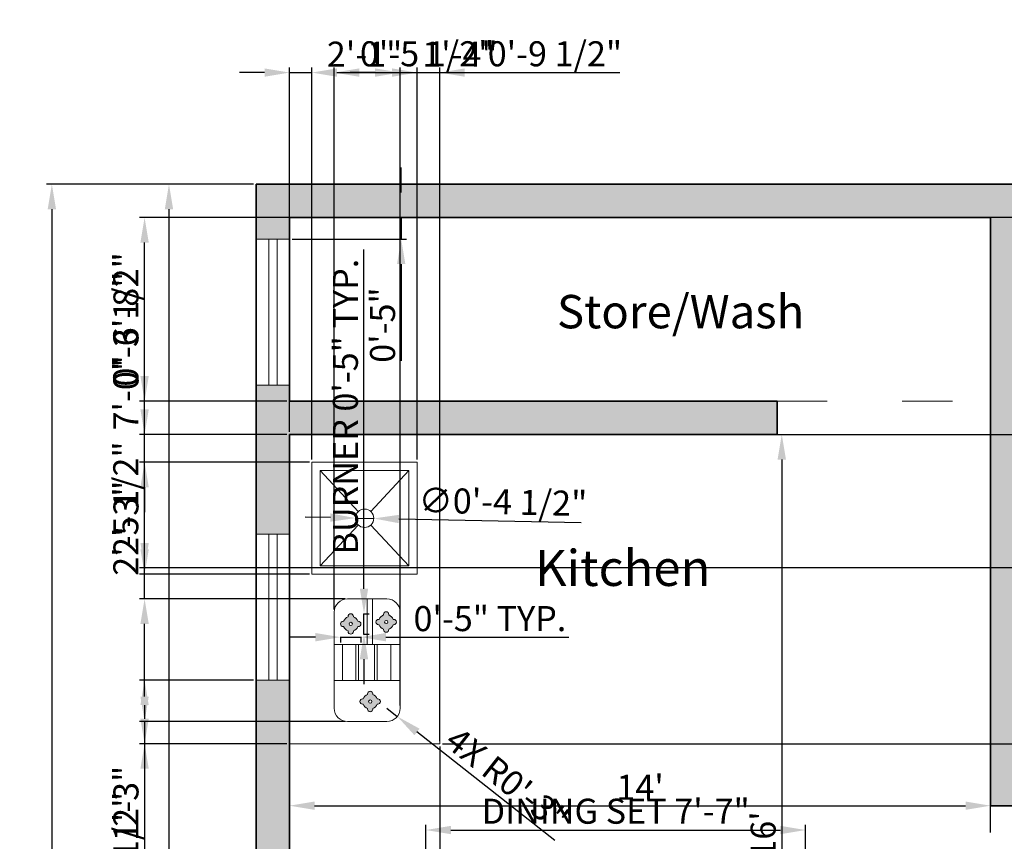
# Model space of a CAD drawing. Units: inches. Extents: x 2129 to 3258, y 1851 to 3021.
# Tile 6 of 10: x 2129 to 2365, y 2250 to 2447. Entities that reach past the tile are written whole.
import ezdxf

# ---------------------------------------------------------------- set-up
doc = ezdxf.new("R2010")
doc.units = ezdxf.units.IN
doc.linetypes.add('ACAD_ISO03W100', pattern=[30, 12, -18])
for name, color, linetype, lineweight in [('A-ANNO-DIMS', 2, 'Continuous', 18), ('A-AREA-IDEN', 7, 'Continuous', 20), ('A-EQPM', 4, 'Continuous', 13), ('A-FLOR-CASE', 8, 'Continuous', 18), ('A-FLOR-FIXT', 9, 'Continuous', 18), ('A-GLAZ', 4, 'Continuous', 18), ('A-WALL', 7, 'Continuous', 35), ('A-WALL-OVHD', 8, 'ACAD_ISO03W100', 18)]:
    doc.layers.add(name, color=color, linetype=linetype, lineweight=lineweight)
doc.layers.add('A-WALL-PATT', color=32, linetype='Continuous', lineweight=13, true_color=0xcd6928)
doc.styles.get("Standard").update_dxf_attribs({"font": 'arial.ttf'})
doc.dimstyles.new('ISO-25', dxfattribs={"dimtxt": 6, "dimasz": 6, "dimexe": 1.25, "dimexo": 0.625, "dimtad": 1, "dimdec": 1, "dimlunit": 3, "dimtxsty": 'Standard', "dimcen": 2.5, "dimclrd": 5, "dimclre": 5, "dimadec": 0, "dimazin": 0, "dimtfac": 1, "dimtdec": 1, "dimtmove": 0, "dimatfit": 3, "dimfxl": 1, "dimarcsym": 0})

# ---------------------------------------------------------------- blocks, each defined once
blk = doc.blocks.new('*D5')
at = {"layer": 'A-ANNO-DIMS', "color": 0, "lineweight": -2, "transparency": 16777216}
for p, q in [((2185.3, 2407.23), (2163.77, 2407.23)), ((2165.02, 2401.23), (2165.02, 1965.23)), ((2185.3, 1959.23), (2163.77, 1959.23))]:
    blk.add_line(p, q, dxfattribs=at)
at = {"layer": 'A-ANNO-DIMS', "color": 0, "transparency": 16777216}
for points in [[(2164.02, 2401.23), (2166.02, 2401.23), (2165.02, 2407.23)], [(2164.02, 1965.23), (2166.02, 1965.23), (2165.02, 1959.23)]]:
    blk.add_solid(points, dxfattribs=at)
at = {"layer": 'Defpoints', "color": 0, "transparency": 16777216}
for p in [(2185.93, 2407.23), (2165.02, 1959.23), (2185.93, 1959.23)]:
    blk.add_point(p, dxfattribs=at)
at = {"layer": 'A-ANNO-DIMS', "color": 0, "transparency": 16777216, "insert": (2161.33, 2183.23), "char_height": 6, "attachment_point": 5, "rotation": 90}
blk.add_mtext('37\'-4"', dxfattribs=at)
blk = doc.blocks.new('*D6')
at = {"layer": 'A-ANNO-DIMS', "color": 0, "lineweight": -2, "transparency": 16777216}
for p, q in [((2185.3, 2407.23), (2135.71, 2407.23)), ((2136.96, 2401.23), (2136.96, 1885.23)), ((2185.3, 1879.23), (2135.71, 1879.23))]:
    blk.add_line(p, q, dxfattribs=at)
at = {"layer": 'A-ANNO-DIMS', "color": 0, "transparency": 16777216}
for points in [[(2135.96, 2401.23), (2137.96, 2401.23), (2136.96, 2407.23)], [(2135.96, 1885.23), (2137.96, 1885.23), (2136.96, 1879.23)]]:
    blk.add_solid(points, dxfattribs=at)
at = {"layer": 'Defpoints', "color": 0, "transparency": 16777216}
for p in [(2185.93, 2407.23), (2136.96, 1879.23), (2185.93, 1879.23)]:
    blk.add_point(p, dxfattribs=at)
at = {"layer": 'A-ANNO-DIMS', "color": 0, "transparency": 16777216, "insert": (2133.34, 2143.23), "char_height": 6, "attachment_point": 5, "rotation": 90}
blk.add_mtext("44'", dxfattribs=at)
blk = doc.blocks.new('*D7')
at = {"layer": 'A-ANNO-DIMS', "color": 0, "lineweight": -2, "transparency": 16777216}
for p, q in [((2311.4, 2347.23), (2313.14, 2347.23)), ((2311.89, 2341.23), (2311.89, 2161.23)), ((2311.4, 2155.23), (2313.14, 2155.23))]:
    blk.add_line(p, q, dxfattribs=at)
at = {"layer": 'A-ANNO-DIMS', "color": 0, "transparency": 16777216}
for points in [[(2310.89, 2341.23), (2312.89, 2341.23), (2311.89, 2347.23)], [(2310.89, 2161.23), (2312.89, 2161.23), (2311.89, 2155.23)]]:
    blk.add_solid(points, dxfattribs=at)
at = {"layer": 'Defpoints', "color": 0, "transparency": 16777216}
for p in [(2310.77, 2347.23), (2310.77, 2155.23), (2311.89, 2155.23)]:
    blk.add_point(p, dxfattribs=at)
at = {"layer": 'A-ANNO-DIMS', "color": 0, "transparency": 16777216, "insert": (2308.2, 2251.23), "char_height": 6, "attachment_point": 5, "rotation": 90}
blk.add_mtext("16'", dxfattribs=at)
blk = doc.blocks.new('*D8')
at = {"layer": 'A-ANNO-DIMS', "color": 0, "lineweight": -2, "transparency": 16777216}
for p, q in [((2193.93, 2251.86), (2193.93, 2259.5)), ((2361.93, 2251.86), (2361.93, 2259.5)), ((2199.93, 2258.25), (2355.93, 2258.25))]:
    blk.add_line(p, q, dxfattribs=at)
at = {"layer": 'A-ANNO-DIMS', "color": 0, "transparency": 16777216}
for points in [[(2199.93, 2259.25), (2199.93, 2257.25), (2193.93, 2258.25)], [(2355.93, 2259.25), (2355.93, 2257.25), (2361.93, 2258.25)]]:
    blk.add_solid(points, dxfattribs=at)
at = {"layer": 'Defpoints', "color": 0, "transparency": 16777216}
for p in [(2361.93, 2258.25), (2193.93, 2251.23), (2361.93, 2251.23)]:
    blk.add_point(p, dxfattribs=at)
at = {"layer": 'A-ANNO-DIMS', "color": 0, "transparency": 16777216, "insert": (2277.93, 2261.89), "char_height": 6, "attachment_point": 5}
blk.add_mtext("14'", dxfattribs=at)
blk = doc.blocks.new('WIN-PLAN-35')
for p, q in [((0, 5), (35, 5)), ((0, 3), (35, 3))]:
    blk.add_line(p, q)
blk.add_lwpolyline([(0, 8), (35, 8), (35, 0), (0, 0)], close=True)
blk = doc.blocks.new('COOKTOP-BURNER')
h = blk.add_hatch(color=256)
h.dxf.hatch_style = 1
h.paths.add_polyline_path([(0.76, 3.09), (0.64, 3.09, 1), (0.64, 1.81), (0.76, 1.81, 0.214506), (1.81, 0.76), (1.81, 0.64, 1), (3.09, 0.64), (3.09, 0.76, 0.214506), (4.14, 1.81), (4.26, 1.81, 1), (4.26, 3.09), (4.14, 3.09, 0.214506), (3.09, 4.14), (3.09, 4.26, 1), (1.81, 4.26), (1.81, 4.14, 0.214506)])
h.paths.add_polyline_path([(2.45, 2.84, -1), (2.45, 2.06, -1)], flags=16)
for p, q in [((0.64, 3.09), (0.76, 3.09)), ((1.81, 4.14), (1.81, 4.26)), ((3.09, 4.14), (3.09, 4.26)), ((4.14, 3.09), (4.26, 3.09)), ((0.64, 1.81), (0.76, 1.81)), ((1.81, 0.64), (1.81, 0.76)), ((3.09, 0.64), (3.09, 0.76)), ((4.14, 1.81), (4.26, 1.81))]:
    blk.add_line(p, q)
blk.add_circle((2.45, 2.45), 0.392)
for centre, radius, start, end in [((2.45, 4.26), 0.642, 0, 180), ((0.64, 2.45), 0.642, 90, 270), ((2.45, 2.45), 1.81, 110.7864, 159.2136), ((2.45, 2.45), 1.81, 20.7864, 69.2136), ((4.26, 2.45), 0.642, 270, 90), ((2.45, 2.45), 1.81, 200.7864, 249.2136), ((2.45, 0.64), 0.642, 180, 0), ((2.45, 2.45), 1.81, 290.7864, 339.2136)]:
    blk.add_arc(centre, radius, start, end)
blk = doc.blocks.new('*D70')
at = {"layer": 'A-ANNO-DIMS', "color": 5, "lineweight": -2, "transparency": 16777216}
for p, q in [((2211.76, 2310.27), (2211.76, 2391.55)), ((2211.65, 2304.27), (2213.01, 2304.27)), ((2211.76, 2299.37), (2211.76, 2304.27)), ((2211.65, 2299.37), (2213.01, 2299.37)), ((2211.76, 2293.37), (2211.76, 2287.37))]:
    blk.add_line(p, q, dxfattribs=at)
at = {"layer": 'A-ANNO-DIMS', "color": 5, "transparency": 16777216}
for points in [[(2210.76, 2310.27), (2212.76, 2310.27), (2211.76, 2304.27)], [(2210.76, 2293.37), (2212.76, 2293.37), (2211.76, 2299.37)]]:
    blk.add_solid(points, dxfattribs=at)
at = {"layer": 'Defpoints', "color": 0, "transparency": 16777216}
for p in [(2211.03, 2304.27), (2211.76, 2304.27), (2211.03, 2299.37)]:
    blk.add_point(p, dxfattribs=at)
at = {"layer": 'A-ANNO-DIMS', "color": 0, "transparency": 16777216, "insert": (2208.08, 2353.91), "char_height": 6, "attachment_point": 5, "rotation": 90}
blk.add_mtext('BURNER 0\'-5" TYP.', dxfattribs=at)
blk = doc.blocks.new('*D71')
at = {"layer": 'A-ANNO-DIMS', "color": 5, "lineweight": -2, "transparency": 16777216}
for p, q in [((2200.13, 2298.64), (2194.13, 2298.64)), ((2206.13, 2298.75), (2206.13, 2297.39)), ((2206.13, 2298.64), (2211.03, 2298.64)), ((2211.03, 2298.75), (2211.03, 2297.39)), ((2217.03, 2298.64), (2260.85, 2298.64))]:
    blk.add_line(p, q, dxfattribs=at)
at = {"layer": 'A-ANNO-DIMS', "color": 5, "transparency": 16777216}
for points in [[(2200.13, 2299.64), (2200.13, 2297.64), (2206.13, 2298.64)], [(2217.03, 2299.64), (2217.03, 2297.64), (2211.03, 2298.64)]]:
    blk.add_solid(points, dxfattribs=at)
at = {"layer": 'Defpoints', "color": 0, "transparency": 16777216}
for p in [(2206.13, 2299.37), (2211.03, 2299.37), (2211.03, 2298.64)]:
    blk.add_point(p, dxfattribs=at)
at = {"layer": 'A-ANNO-DIMS', "color": 0, "transparency": 16777216, "insert": (2241.94, 2302.32), "char_height": 6, "attachment_point": 5}
blk.add_mtext('0\'-5" TYP.', dxfattribs=at)
blk = doc.blocks.new('*D78')
at = {"layer": 'A-ANNO-DIMS', "color": 5, "lineweight": -2, "transparency": 16777216}
for p, q in [((2226.58, 2239.39), (2226.58, 2253.67)), ((2317.58, 2239.39), (2317.58, 2253.67)), ((2232.58, 2252.42), (2311.58, 2252.42))]:
    blk.add_line(p, q, dxfattribs=at)
at = {"layer": 'A-ANNO-DIMS', "color": 5, "transparency": 16777216}
for points in [[(2232.58, 2253.42), (2232.58, 2251.42), (2226.58, 2252.42)], [(2311.58, 2253.42), (2311.58, 2251.42), (2317.58, 2252.42)]]:
    blk.add_solid(points, dxfattribs=at)
at = {"layer": 'Defpoints', "color": 0, "transparency": 16777216}
for p in [(2317.58, 2252.42), (2226.58, 2238.77), (2317.58, 2238.77)]:
    blk.add_point(p, dxfattribs=at)
at = {"layer": 'A-ANNO-DIMS', "color": 0, "transparency": 16777216, "insert": (2272.08, 2256.15), "char_height": 6, "attachment_point": 5}
blk.add_mtext('DINING SET 7\'-7"', dxfattribs=at)
blk = doc.blocks.new('*D92')
at = {"layer": 'A-ANNO-DIMS', "color": 5, "lineweight": -2, "transparency": 16777216}
for p, q in [((2369.3, 2399.23), (2157.93, 2399.23)), ((2159.18, 2321.23), (2159.18, 2393.23)), ((2369.3, 2315.23), (2157.93, 2315.23))]:
    blk.add_line(p, q, dxfattribs=at)
at = {"layer": 'A-ANNO-DIMS', "color": 5, "transparency": 16777216}
for points in [[(2158.18, 2393.23), (2160.18, 2393.23), (2159.18, 2399.23)], [(2158.18, 2321.23), (2160.18, 2321.23), (2159.18, 2315.23)]]:
    blk.add_solid(points, dxfattribs=at)
at = {"layer": 'Defpoints', "color": 0, "transparency": 16777216}
for p in [(2159.18, 2399.23), (2369.93, 2399.23), (2369.93, 2315.23)]:
    blk.add_point(p, dxfattribs=at)
at = {"layer": 'A-ANNO-DIMS', "color": 0, "transparency": 16777216, "insert": (2155.49, 2357.23), "char_height": 6, "attachment_point": 5, "rotation": 90}
blk.add_mtext('7\'-0"', dxfattribs=at)
blk = doc.blocks.new('*D93')
at = {"layer": 'A-ANNO-DIMS', "color": 5, "lineweight": -2, "transparency": 16777216}
for p, q in [((2193.3, 2399.23), (2157.93, 2399.23)), ((2159.18, 2361.23), (2159.18, 2393.23)), ((2193.3, 2355.23), (2157.93, 2355.23))]:
    blk.add_line(p, q, dxfattribs=at)
at = {"layer": 'A-ANNO-DIMS', "color": 5, "transparency": 16777216}
for points in [[(2158.18, 2393.23), (2160.18, 2393.23), (2159.18, 2399.23)], [(2158.18, 2361.23), (2160.18, 2361.23), (2159.18, 2355.23)]]:
    blk.add_solid(points, dxfattribs=at)
at = {"layer": 'Defpoints', "color": 0, "transparency": 16777216}
for p in [(2159.18, 2399.23), (2193.93, 2399.23), (2193.93, 2355.23)]:
    blk.add_point(p, dxfattribs=at)
at = {"layer": 'A-ANNO-DIMS', "color": 0, "transparency": 16777216, "insert": (2155.49, 2377.23), "char_height": 6, "attachment_point": 5, "rotation": 90}
blk.add_mtext('3\'-8"', dxfattribs=at)
blk = doc.blocks.new('*D97')
at = {"layer": 'A-ANNO-DIMS', "color": 5, "lineweight": -2, "transparency": 16777216}
for p, q in [((2193.93, 2272.48), (2193.93, 1851.23)), ((2229.93, 2272.48), (2229.93, 1851.23)), ((2199.93, 1852.48), (2223.93, 1852.48))]:
    blk.add_line(p, q, dxfattribs=at)
at = {"layer": 'A-ANNO-DIMS', "color": 5, "transparency": 16777216}
for points in [[(2199.93, 1853.48), (2199.93, 1851.48), (2193.93, 1852.48)], [(2223.93, 1853.48), (2223.93, 1851.48), (2229.93, 1852.48)]]:
    blk.add_solid(points, dxfattribs=at)
at = {"layer": 'Defpoints', "color": 0, "transparency": 16777216}
for p in [(2193.93, 2273.1), (2229.93, 2273.1), (2229.93, 1852.48)]:
    blk.add_point(p, dxfattribs=at)
at = {"layer": 'A-ANNO-DIMS', "color": 0, "transparency": 16777216, "insert": (2211.93, 1856.18), "char_height": 6, "attachment_point": 5}
blk.add_mtext('3\'-0"', dxfattribs=at)
blk = doc.blocks.new('*D98')
at = {"layer": 'A-ANNO-DIMS', "color": 5, "lineweight": -2, "transparency": 16777216}
for p, q in [((2230.55, 2347.23), (2597.93, 2347.23)), ((2596.68, 2279.1), (2596.68, 2341.23)), ((2230.55, 2273.1), (2597.93, 2273.1))]:
    blk.add_line(p, q, dxfattribs=at)
at = {"layer": 'A-ANNO-DIMS', "color": 5, "transparency": 16777216}
for points in [[(2595.68, 2341.23), (2597.68, 2341.23), (2596.68, 2347.23)], [(2595.68, 2279.1), (2597.68, 2279.1), (2596.68, 2273.1)]]:
    blk.add_solid(points, dxfattribs=at)
at = {"layer": 'Defpoints', "color": 0, "transparency": 16777216}
for p in [(2229.93, 2347.23), (2596.68, 2347.23), (2229.93, 2273.1)]:
    blk.add_point(p, dxfattribs=at)
at = {"layer": 'A-ANNO-DIMS', "color": 0, "transparency": 16777216, "insert": (2592.99, 2310.17), "char_height": 6, "attachment_point": 5, "rotation": 90}
blk.add_mtext('6\'-2"', dxfattribs=at)
blk = doc.blocks.new('*D99')
at = {"layer": 'A-ANNO-DIMS', "color": 5, "lineweight": -2, "transparency": 16777216}
for p, q in [((2199.29, 2341.21), (2199.29, 2435.23)), ((2205.29, 2433.98), (2218.51, 2433.98)), ((2224.51, 2341.21), (2224.51, 2435.23))]:
    blk.add_line(p, q, dxfattribs=at)
at = {"layer": 'A-ANNO-DIMS', "color": 5, "transparency": 16777216}
for points in [[(2205.29, 2434.98), (2205.29, 2432.98), (2199.29, 2433.98)], [(2218.51, 2434.98), (2218.51, 2432.98), (2224.51, 2433.98)]]:
    blk.add_solid(points, dxfattribs=at)
at = {"layer": 'Defpoints', "color": 0, "transparency": 16777216}
for p in [(2224.51, 2433.98), (2199.29, 2340.59), (2224.51, 2340.59)]:
    blk.add_point(p, dxfattribs=at)
at = {"layer": 'A-ANNO-DIMS', "color": 0, "transparency": 16777216, "insert": (2211.9, 2437.62), "char_height": 6, "attachment_point": 5}
blk.add_mtext('2\'-1"', dxfattribs=at)
blk = doc.blocks.new('*D100')
at = {"layer": 'A-ANNO-DIMS', "color": 5, "lineweight": -2, "transparency": 16777216}
for p, q in [((2198.67, 2340.59), (2157.93, 2340.59)), ((2159.18, 2319.71), (2159.18, 2334.59)), ((2198.67, 2313.71), (2157.93, 2313.71))]:
    blk.add_line(p, q, dxfattribs=at)
at = {"layer": 'A-ANNO-DIMS', "color": 5, "transparency": 16777216}
for points in [[(2158.18, 2334.59), (2160.18, 2334.59), (2159.18, 2340.59)], [(2158.18, 2319.71), (2160.18, 2319.71), (2159.18, 2313.71)]]:
    blk.add_solid(points, dxfattribs=at)
at = {"layer": 'Defpoints', "color": 0, "transparency": 16777216}
for p in [(2159.18, 2340.59), (2199.29, 2340.59), (2199.29, 2313.71)]:
    blk.add_point(p, dxfattribs=at)
at = {"layer": 'A-ANNO-DIMS', "color": 0, "transparency": 16777216, "insert": (2155.49, 2327.15), "char_height": 6, "attachment_point": 5, "rotation": 90}
blk.add_mtext('2\'-3"', dxfattribs=at)
blk = doc.blocks.new('*D101')
at = {"layer": 'A-ANNO-DIMS', "color": 5, "lineweight": -2, "transparency": 16777216}
for p, q in [((2204.64, 2305.25), (2204.64, 2435.23)), ((2210.64, 2433.98), (2214.44, 2433.98)), ((2220.44, 2305.25), (2220.44, 2435.23)), ((2220.44, 2433.98), (2243.07, 2433.98))]:
    blk.add_line(p, q, dxfattribs=at)
at = {"layer": 'A-ANNO-DIMS', "color": 5, "transparency": 16777216}
for points in [[(2210.64, 2434.98), (2210.64, 2432.98), (2204.64, 2433.98)], [(2214.44, 2434.98), (2214.44, 2432.98), (2220.44, 2433.98)]]:
    blk.add_solid(points, dxfattribs=at)
at = {"layer": 'Defpoints', "color": 0, "transparency": 16777216}
for p in [(2220.44, 2433.98), (2204.64, 2304.63), (2220.44, 2304.63)]:
    blk.add_point(p, dxfattribs=at)
at = {"layer": 'A-ANNO-DIMS', "color": 0, "transparency": 16777216, "insert": (2234.76, 2437.62), "char_height": 6, "attachment_point": 5}
blk.add_mtext('1\'-4"', dxfattribs=at)
blk = doc.blocks.new('*D102')
at = {"layer": 'A-ANNO-DIMS', "color": 5, "lineweight": -2, "transparency": 16777216}
for p, q in [((2159.18, 2307.84), (2159.18, 2345.12)), ((2207.23, 2307.84), (2157.93, 2307.84)), ((2159.18, 2284.42), (2159.18, 2301.84)), ((2207.23, 2278.42), (2157.93, 2278.42))]:
    blk.add_line(p, q, dxfattribs=at)
at = {"layer": 'A-ANNO-DIMS', "color": 5, "transparency": 16777216}
for points in [[(2158.18, 2301.84), (2160.18, 2301.84), (2159.18, 2307.84)], [(2158.18, 2284.42), (2160.18, 2284.42), (2159.18, 2278.42)]]:
    blk.add_solid(points, dxfattribs=at)
at = {"layer": 'Defpoints', "color": 0, "transparency": 16777216}
for p in [(2159.18, 2307.84), (2207.85, 2307.84), (2207.85, 2278.42)]:
    blk.add_point(p, dxfattribs=at)
at = {"layer": 'A-ANNO-DIMS', "color": 0, "transparency": 16777216, "insert": (2155.45, 2329.48), "char_height": 6, "attachment_point": 5, "rotation": 90}
blk.add_mtext('2\'-5 1/2"', dxfattribs=at)
blk = doc.blocks.new('*D103')
at = {"layer": 'A-ANNO-DIMS', "color": 5, "lineweight": -2, "transparency": 16777216}
for p, q in [((2187.93, 2433.98), (2181.93, 2433.98)), ((2193.93, 2347.86), (2193.93, 2435.23)), ((2193.93, 2433.98), (2199.29, 2433.98)), ((2199.29, 2341.21), (2199.29, 2435.23)), ((2205.29, 2433.98), (2242.47, 2433.98))]:
    blk.add_line(p, q, dxfattribs=at)
at = {"layer": 'A-ANNO-DIMS', "color": 5, "transparency": 16777216}
for points in [[(2187.93, 2434.98), (2187.93, 2432.98), (2193.93, 2433.98)], [(2205.29, 2434.98), (2205.29, 2432.98), (2199.29, 2433.98)]]:
    blk.add_solid(points, dxfattribs=at)
at = {"layer": 'Defpoints', "color": 0, "transparency": 16777216}
for p in [(2199.29, 2433.98), (2193.93, 2347.23), (2199.29, 2340.59)]:
    blk.add_point(p, dxfattribs=at)
at = {"layer": 'A-ANNO-DIMS', "color": 0, "transparency": 16777216, "insert": (2226.88, 2437.71), "char_height": 6, "attachment_point": 5}
blk.add_mtext('0\'-5 1/2"', dxfattribs=at)
blk = doc.blocks.new('*D104')
at = {"layer": 'A-ANNO-DIMS', "color": 5, "lineweight": -2, "transparency": 16777216}
for p, q in [((2159.18, 2353.23), (2159.18, 2390.42)), ((2193.3, 2347.23), (2157.93, 2347.23)), ((2159.18, 2340.59), (2159.18, 2347.23)), ((2198.67, 2340.59), (2157.93, 2340.59)), ((2159.18, 2334.59), (2159.18, 2328.59))]:
    blk.add_line(p, q, dxfattribs=at)
at = {"layer": 'A-ANNO-DIMS', "color": 5, "transparency": 16777216}
for points in [[(2158.18, 2353.23), (2160.18, 2353.23), (2159.18, 2347.23)], [(2158.18, 2334.59), (2160.18, 2334.59), (2159.18, 2340.59)]]:
    blk.add_solid(points, dxfattribs=at)
at = {"layer": 'Defpoints', "color": 0, "transparency": 16777216}
for p in [(2159.18, 2347.23), (2193.93, 2347.23), (2199.29, 2340.59)]:
    blk.add_point(p, dxfattribs=at)
at = {"layer": 'A-ANNO-DIMS', "color": 0, "transparency": 16777216, "insert": (2155.45, 2374.82), "char_height": 6, "attachment_point": 5, "rotation": 90}
blk.add_mtext('0\'-6 1/2"', dxfattribs=at)
blk = doc.blocks.new('*D105')
at = {"layer": 'A-ANNO-DIMS', "color": 5, "lineweight": -2, "transparency": 16777216}
for p, q in [((2214.44, 2433.98), (2208.44, 2433.98)), ((2220.44, 2282.25), (2220.44, 2435.23)), ((2220.44, 2433.98), (2229.93, 2433.98)), ((2229.93, 2273.73), (2229.93, 2435.23)), ((2235.93, 2433.98), (2273.11, 2433.98))]:
    blk.add_line(p, q, dxfattribs=at)
at = {"layer": 'A-ANNO-DIMS', "color": 5, "transparency": 16777216}
for points in [[(2214.44, 2434.98), (2214.44, 2432.98), (2220.44, 2433.98)], [(2235.93, 2434.98), (2235.93, 2432.98), (2229.93, 2433.98)]]:
    blk.add_solid(points, dxfattribs=at)
at = {"layer": 'Defpoints', "color": 0, "transparency": 16777216}
for p in [(2229.93, 2433.98), (2220.44, 2281.62), (2229.93, 2273.1)]:
    blk.add_point(p, dxfattribs=at)
at = {"layer": 'A-ANNO-DIMS', "color": 0, "transparency": 16777216, "insert": (2257.52, 2437.71), "char_height": 6, "attachment_point": 5}
blk.add_mtext('0\'-9 1/2"', dxfattribs=at)
blk = doc.blocks.new('*D106')
at = {"layer": 'A-ANNO-DIMS', "color": 5, "lineweight": -2, "transparency": 16777216}
for p, q in [((2159.18, 2284.42), (2159.18, 2290.42)), ((2207.23, 2278.42), (2157.93, 2278.42)), ((2159.18, 2278.42), (2159.18, 2273.1)), ((2193.3, 2273.1), (2157.93, 2273.1)), ((2159.18, 2267.1), (2159.18, 2229.92))]:
    blk.add_line(p, q, dxfattribs=at)
at = {"layer": 'A-ANNO-DIMS', "color": 5, "transparency": 16777216}
for points in [[(2158.18, 2284.42), (2160.18, 2284.42), (2159.18, 2278.42)], [(2158.18, 2267.1), (2160.18, 2267.1), (2159.18, 2273.1)]]:
    blk.add_solid(points, dxfattribs=at)
at = {"layer": 'Defpoints', "color": 0, "transparency": 16777216}
for p in [(2207.85, 2278.42), (2159.18, 2273.1), (2193.93, 2273.1)]:
    blk.add_point(p, dxfattribs=at)
at = {"layer": 'A-ANNO-DIMS', "color": 0, "transparency": 16777216, "insert": (2155.45, 2245.51), "char_height": 6, "attachment_point": 5, "rotation": 90}
blk.add_mtext('0\'-5 1/2"', dxfattribs=at)
blk = doc.blocks.new('*D108')
at = {"layer": 'A-ANNO-DIMS', "color": 5, "lineweight": -2, "transparency": 16777216}
for p, q in [((2220.68, 2405.23), (2220.68, 2411.23)), ((2194.55, 2399.23), (2221.93, 2399.23)), ((2220.68, 2399.23), (2220.68, 2394.06)), ((2194.55, 2394.06), (2221.93, 2394.06)), ((2220.68, 2388.06), (2220.68, 2364.86))]:
    blk.add_line(p, q, dxfattribs=at)
at = {"layer": 'A-ANNO-DIMS', "color": 5, "transparency": 16777216}
for points in [[(2219.68, 2405.23), (2221.68, 2405.23), (2220.68, 2399.23)], [(2219.68, 2388.06), (2221.68, 2388.06), (2220.68, 2394.06)]]:
    blk.add_solid(points, dxfattribs=at)
at = {"layer": 'Defpoints', "color": 0, "transparency": 16777216}
for p in [(2193.93, 2399.23), (2193.93, 2394.06), (2220.68, 2394.06)]:
    blk.add_point(p, dxfattribs=at)
at = {"layer": 'A-ANNO-DIMS', "color": 0, "transparency": 16777216, "insert": (2216.99, 2373.46), "char_height": 6, "attachment_point": 5, "rotation": 90}
blk.add_mtext('0\'-5"', dxfattribs=at)
blk = doc.blocks.new('*D109')
at = {"layer": 'A-ANNO-DIMS', "color": 5, "lineweight": -2, "transparency": 16777216}
for p, q in [((2185.3, 2288.35), (2157.93, 2288.35)), ((2159.18, 2282.35), (2159.18, 2279.1)), ((2193.3, 2273.1), (2157.93, 2273.1)), ((2159.18, 2273.1), (2159.18, 2250.47))]:
    blk.add_line(p, q, dxfattribs=at)
at = {"layer": 'A-ANNO-DIMS', "color": 5, "transparency": 16777216}
for points in [[(2158.18, 2282.35), (2160.18, 2282.35), (2159.18, 2288.35)], [(2158.18, 2279.1), (2160.18, 2279.1), (2159.18, 2273.1)]]:
    blk.add_solid(points, dxfattribs=at)
at = {"layer": 'Defpoints', "color": 0, "transparency": 16777216}
for p in [(2185.93, 2288.35), (2159.18, 2273.1), (2193.93, 2273.1)]:
    blk.add_point(p, dxfattribs=at)
at = {"layer": 'A-ANNO-DIMS', "color": 0, "transparency": 16777216, "insert": (2155.49, 2258.79), "char_height": 6, "attachment_point": 5, "rotation": 90}
blk.add_mtext('1\'-3"', dxfattribs=at)
blk = doc.blocks.new('*D133')
at = {"layer": 'A-ANNO-DIMS', "color": 5, "lineweight": -2, "transparency": 16777216}
for p, q in [((2203.7, 2327.32), (2197.7, 2327.45)), ((2209.7, 2327.19), (2214.11, 2327.1)), ((2263.8, 2326.04), (2220.11, 2326.97))]:
    blk.add_line(p, q, dxfattribs=at)
at = {"layer": 'A-ANNO-DIMS', "color": 5, "transparency": 16777216}
for points in [[(2203.72, 2328.32), (2203.68, 2326.32), (2209.7, 2327.19)], [(2220.13, 2327.97), (2220.08, 2325.97), (2214.11, 2327.1)]]:
    blk.add_solid(points, dxfattribs=at)
at = {"layer": 'Defpoints', "color": 0, "transparency": 16777216}
for p in [(2209.7, 2327.19), (2214.11, 2327.1)]:
    blk.add_point(p, dxfattribs=at)
at = {"layer": 'A-ANNO-DIMS', "color": 0, "transparency": 16777216, "insert": (2245.04, 2330.3), "char_height": 6, "attachment_point": 5, "rotation": 358.7825}
blk.add_mtext('∅0\'-4 1/2"', dxfattribs=at)
blk = doc.blocks.new('*D134')
at = {"layer": 'A-ANNO-DIMS', "color": 5, "lineweight": -2, "transparency": 16777216}
for p, q in [((2217.23, 2281.62), (2219.75, 2279.64)), ((2257.52, 2249.89), (2224.46, 2275.93))]:
    blk.add_line(p, q, dxfattribs=at)
at = {"layer": 'A-ANNO-DIMS', "color": 5, "transparency": 16777216}
blk.add_solid([(2225.08, 2276.71), (2223.85, 2275.14), (2219.75, 2279.64)], dxfattribs=at)
at = {"layer": 'Defpoints', "color": 0, "transparency": 16777216}
for p in [(2217.23, 2281.62), (2219.75, 2279.64)]:
    blk.add_point(p, dxfattribs=at)
at = {"layer": 'A-ANNO-DIMS', "color": 0, "transparency": 16777216, "insert": (2245.63, 2263.95), "char_height": 6, "attachment_point": 5, "rotation": 321.7707}
blk.add_mtext('4X R0\'-3"', dxfattribs=at)

msp = doc.modelspace()

# ---------------------------------------------------------------- hatches: boundary and pattern name
at = {"layer": 'A-WALL-PATT'}
h = msp.add_hatch(color=256, dxfattribs=at)
h.dxf.hatch_style = 1
h.paths.add_polyline_path([(2393.39, 2407.23), (2185.93, 2407.23), (2185.93, 2394.06), (2193.93, 2394.06), (2193.93, 2399.23), (2361.93, 2399.23), (2361.93, 2355.23), (2361.93, 2347.23), (2361.93, 2258.25), (2369.93, 2258.25), (2369.93, 2307.23), (2429.93, 2307.23), (2429.93, 2303.23), (2437.93, 2303.23), (2437.93, 2327.23), (2429.93, 2327.23), (2429.93, 2315.23), (2369.93, 2315.23), (2369.93, 2399.23), (2393.39, 2399.23)])
h.paths.add_polyline_path([(2569.93, 2407.23), (2410.42, 2407.23), (2410.42, 2399.23), (2429.93, 2399.23), (2429.93, 2351.23), (2437.93, 2351.23), (2437.93, 2399.23), (2561.93, 2399.23), (2561.93, 2317.22), (2569.93, 2317.22)])
h.paths.add_polyline_path([(2569.93, 2282.22), (2561.93, 2282.22), (2561.93, 2243.23), (2437.93, 2243.23), (2437.93, 2249.23), (2429.93, 2249.23), (2429.93, 2235.23), (2561.93, 2235.23), (2561.93, 2155.23), (2379.93, 2155.23), (2379.93, 2147.23), (2385.93, 2147.23), (2385.93, 2141.23), (2393.93, 2141.23), (2393.93, 2147.23), (2469.93, 2147.23), (2469.93, 2111.23), (2477.93, 2111.23), (2477.93, 2147.23), (2561.93, 2147.23), (2561.93, 2129.53), (2569.93, 2129.53)])
h.paths.add_polyline_path([(2569.93, 2112.5), (2561.93, 2112.5), (2561.93, 2063.23), (2477.93, 2063.23), (2477.93, 2069.23), (2469.93, 2069.23), (2469.93, 2063.23), (2445.93, 2063.23), (2445.93, 2055.23), (2561.93, 2055.23), (2561.93, 1951.04), (2569.93, 1951.04)])
h.paths.add_polyline_path([(2569.93, 1916.04), (2561.93, 1916.04), (2561.93, 1887.23), (2393.93, 1887.23), (2393.93, 2055.23), (2399.93, 2055.23), (2399.93, 2063.23), (2393.93, 2063.23), (2393.93, 2087.23), (2385.93, 2087.23), (2385.93, 1887.23), (2385.93, 1879.23), (2569.93, 1879.23)])
h.paths.add_polyline_path([(2193.93, 2147.23), (2289.93, 2147.23), (2289.93, 2155.23), (2193.93, 2155.23), (2193.93, 2170.77), (2185.93, 2170.77), (2185.93, 2056.85), (2193.93, 2056.85)])
h.paths.add_polyline_path([(2193.93, 2021.85), (2185.93, 2021.85), (2185.93, 1959.23), (2222.56, 1959.23), (2222.56, 1967.23), (2193.93, 1967.23)])
h.paths.add_polyline_path([(2307.93, 1967.23), (2257.56, 1967.23), (2257.56, 1959.23), (2307.93, 1959.23)])
h.paths.add_polyline_path([(2255.61, 2368.18), (2321.09, 2368.18), (2321.09, 2384.66), (2255.61, 2384.66)], flags=25)
h.paths.add_polyline_path([(2282.89, 2032.34), (2325.27, 2032.34), (2325.27, 2051.27), (2282.89, 2051.27)], flags=9)
h.paths.add_polyline_path([(2404.09, 1945.18), (2463.36, 1945.18), (2463.36, 1961.66), (2404.09, 1961.66)], flags=25)
h.paths.add_polyline_path([(2494.41, 2286.84), (2553.68, 2286.84), (2553.68, 2303.32), (2494.41, 2303.32)], flags=9)
h.paths.add_polyline_path([(2389.71, 2321.98), (2411.09, 2321.98), (2411.09, 2338.47), (2389.71, 2338.47)], flags=25)
h.paths.add_polyline_path([(2219.41, 2162.82), (2258.18, 2162.82), (2258.18, 2179.3), (2219.41, 2179.3)], flags=9)
h.paths.add_polyline_path([(2249.68, 2306.23), (2298.12, 2306.23), (2298.12, 2323.98), (2249.68, 2323.98)], flags=25)
h = msp.add_hatch(color=256, dxfattribs=at)
h.dxf.hatch_style = 1
h.paths.add_polyline_path([(2193.93, 2288.35), (2185.93, 2288.35), (2185.93, 2205.77), (2193.93, 2205.77)])
h.paths.add_polyline_path([(2193.93, 2347.23), (2310.77, 2347.23), (2310.77, 2355.23), (2193.93, 2355.23), (2193.93, 2359.06), (2185.93, 2359.06), (2185.93, 2323.35), (2193.93, 2323.35)])
h.paths.add_polyline_path([(2314.44, 2244.01), (2314.44, 2257.94), (2302.07, 2257.94), (2302.07, 2244.01)], flags=9)
h.paths.add_polyline_path([(2255.61, 2368.18), (2321.09, 2368.18), (2321.09, 2384.66), (2255.61, 2384.66)], flags=9)
h.paths.add_polyline_path([(2282.89, 2032.34), (2325.27, 2032.34), (2325.27, 2051.27), (2282.89, 2051.27)], flags=9)
h.paths.add_polyline_path([(2404.09, 1945.18), (2463.36, 1945.18), (2463.36, 1961.66), (2404.09, 1961.66)], flags=9)
h.paths.add_polyline_path([(2494.41, 2286.84), (2553.68, 2286.84), (2553.68, 2303.32), (2494.41, 2303.32)], flags=9)
h.paths.add_polyline_path([(2389.71, 2321.98), (2411.09, 2321.98), (2411.09, 2338.47), (2389.71, 2338.47)], flags=9)
h.paths.add_polyline_path([(2219.41, 2162.82), (2258.18, 2162.82), (2258.18, 2179.3), (2219.41, 2179.3)], flags=9)
h.paths.add_polyline_path([(2249.68, 2306.23), (2298.12, 2306.23), (2298.12, 2323.98), (2249.68, 2323.98)], flags=9)

# ---------------------------------------------------------------- linework, layer by layer
at = {"layer": 'A-EQPM'}
for p, q in [((2207.85, 2307.84), (2217.23, 2307.84)), ((2212.54, 2307.84), (2212.54, 2296.86)), ((2213.82, 2296.86), (2213.82, 2307.84)), ((2204.64, 2281.62), (2204.64, 2304.63)), ((2220.44, 2304.63), (2220.44, 2281.62)), ((2204.64, 2296.86), (2220.44, 2296.86)), ((2206.62, 2288.29), (2206.62, 2296.86)), ((2209.83, 2288.29), (2209.83, 2296.86)), ((2210.47, 2288.29), (2210.47, 2296.86)), ((2214.32, 2288.29), (2214.32, 2296.86)), ((2214.96, 2288.29), (2214.96, 2296.86)), ((2218.17, 2288.29), (2218.17, 2296.86)), ((2212.54, 2288.29), (2204.64, 2288.29)), ((2204.64, 2288.29), (2220.44, 2288.29)), ((2217.23, 2278.42), (2207.85, 2278.42))]:
    msp.add_line(p, q, dxfattribs=at)
for centre, start, end in [((2207.85, 2304.63), 90, 180), ((2217.23, 2304.63), 0, 90), ((2207.85, 2281.62), 180, 270), ((2217.23, 2281.62), 270, 0)]:
    msp.add_arc(centre, 3.21, start, end, dxfattribs=at)
at = {"layer": 'A-FLOR-CASE'}
for p, q in [((2217.93, 2347.23), (2210.52, 2347.23)), ((2210.52, 2347.23), (2217.93, 2347.23)), ((2229.93, 2347.23), (2229.93, 2273.1)), ((2229.93, 2273.1), (2193.93, 2273.1))]:
    msp.add_line(p, q, dxfattribs=at)
at = {"layer": 'A-FLOR-FIXT'}
for p, q in [((2201.29, 2338.59), (2210.4, 2328.76)), ((2222.51, 2338.59), (2213.4, 2328.76)), ((2210.4, 2325.53), (2201.29, 2315.71)), ((2213.4, 2325.53), (2222.51, 2315.71))]:
    msp.add_line(p, q, dxfattribs=at)
for points in [[(2199.29, 2340.59), (2224.51, 2340.59), (2224.51, 2313.71), (2199.29, 2313.71)], [(2201.29, 2338.59), (2222.51, 2338.59), (2222.51, 2315.71), (2201.29, 2315.71)]]:
    msp.add_lwpolyline(points, close=True, dxfattribs=at)
msp.add_circle((2211.9, 2327.15), 2.2, dxfattribs=at)
at = {"layer": 'A-WALL'}
for p, q in [((2361.93, 2399.23), (2361.93, 2355.23)), ((2193.93, 2355.23), (2310.77, 2355.23)), ((2310.77, 2355.23), (2310.77, 2347.23)), ((2361.93, 2355.23), (2361.93, 2347.23)), ((2193.93, 2347.23), (2310.77, 2347.23)), ((2361.93, 2347.23), (2361.93, 2258.25)), ((2361.93, 2258.25), (2369.93, 2258.25))]:
    msp.add_line(p, q, dxfattribs=at)
msp.add_lwpolyline([(2185.93, 2407.23), (2569.93, 2407.23), (2569.93, 1879.23), (2185.93, 1879.23)], close=True, dxfattribs=at)
for points in [[(2193.93, 2355.23), (2193.93, 2399.23), (2361.93, 2399.23)], [(2193.93, 2155.23), (2193.93, 2347.23)]]:
    msp.add_lwpolyline(points, dxfattribs=at)
at = {"layer": 'A-WALL-OVHD'}
for p, q in [((2310.77, 2355.23), (2361.93, 2355.23)), ((2310.77, 2347.23), (2361.93, 2347.23))]:
    msp.add_line(p, q, dxfattribs=at)

# ---------------------------------------------------------------- block references
at = {"layer": 'A-EQPM'}
for p in [(2206.13, 2299.37), (2214.63, 2299.83), (2210.8, 2280.77)]:
    msp.add_blockref('COOKTOP-BURNER', p, dxfattribs=at)
at = {"layer": 'A-GLAZ'}
for p, rotation in [((2185.93, 2394.06), 270.0000000000007), ((2185.93, 2323.35), 270.0000000000009)]:
    msp.add_blockref('WIN-PLAN-35', p, dxfattribs=dict(at, rotation=rotation))

# ---------------------------------------------------------------- texts
at = {"layer": 'A-AREA-IDEN', "attachment_point": 1}
for s, width, gutter_width, heights, insert, char_height in [('{\\fArial|b1|i0|c0|p34;Store/Wash}', 65.2824, 12.5, [0], (2258.02, 2380.68), 8), ('{\\fArial|b1|i0|c0|p34;Kitchen}', 43.7149, 13.46, [8.76], (2252.73, 2319.54), 8.6144)]:
    msp.add_mtext_dynamic_manual_height_columns(s, width=width, gutter_width=gutter_width, heights=heights, dxfattribs=dict(at, insert=insert, char_height=char_height))

# ---------------------------------------------------------------- dimensions: what is measured, and where the dimension line sits
at = {"layer": 'A-ANNO-DIMS'}
for base, p1, p2, override, picture, middle in [((2199.29, 2433.98), (2193.93, 2347.23), (2199.29, 2340.59), {"dimdec": 1, "dimlfac": 1, "dimrnd": 0, "dimzin": 1, "dimdsep": 46, "dimlunit": 4, "dimfrac": 2}, '*D103', (2226.88, 2437.71)), ((2229.93, 2433.98), (2220.44, 2281.62), (2229.93, 2273.1), {"dimdec": 1, "dimlfac": 1, "dimrnd": 0, "dimzin": 1, "dimdsep": 46, "dimlunit": 4, "dimfrac": 2}, '*D105', (2257.52, 2437.71)), ((2224.51, 2433.98), (2199.29, 2340.59), (2224.51, 2340.59), {"dimdec": 1, "dimlfac": 1, "dimrnd": 0, "dimzin": 1, "dimdsep": 46, "dimlunit": 4, "dimfrac": 2}, '*D99', (2211.9, 2437.62)), ((2220.44, 2433.98), (2204.64, 2304.63), (2220.44, 2304.63), {"dimdec": 1, "dimlfac": 1, "dimrnd": 0, "dimzin": 1, "dimdsep": 46, "dimlunit": 4, "dimfrac": 2}, '*D101', (2234.76, 2437.62)), ((2229.93, 1852.48), (2193.93, 2273.1), (2229.93, 2273.1), {"dimdec": 1, "dimlfac": 1, "dimrnd": 0, "dimzin": 1, "dimdsep": 46, "dimlunit": 4, "dimfrac": 2}, '*D97', (2211.93, 1856.18)), ((2361.93, 2258.25), (2193.93, 2251.23), (2361.93, 2251.23), {"dimclrd": 0, "dimclre": 0, "dimclrt": 0}, '*D8', (2277.93, 2261.89))]:
    dim = msp.add_linear_dim(base=base, p1=p1, p2=p2, dimstyle='ISO-25', override=override, dxfattribs=at)
    dim.commit()
    dim.dimension.update_dxf_attribs({"geometry": picture, "text_midpoint": middle})
for base, p1, p2, angle, override, picture, middle in [((2220.68, 2394.06), (2193.93, 2399.23), (2193.93, 2394.06), 270, {"dimdec": 1, "dimlfac": 1, "dimrnd": 0, "dimzin": 1, "dimdsep": 46, "dimlunit": 4, "dimfrac": 2}, '*D108', (2216.99, 2373.46)), ((2136.96, 1879.23), (2185.93, 2407.23), (2185.93, 1879.23), 90, {"dimclrd": 0, "dimclre": 0, "dimclrt": 0}, '*D6', (2133.34, 2143.23)), ((2165.02, 1959.23), (2185.93, 2407.23), (2185.93, 1959.23), 90, {"dimclrd": 0, "dimclre": 0, "dimclrt": 0}, '*D5', (2161.33, 2183.23)), ((2159.18, 2399.23), (2369.93, 2315.23), (2369.93, 2399.23), 90, {"dimdec": 1, "dimlfac": 1, "dimrnd": 0, "dimzin": 1, "dimdsep": 46, "dimlunit": 4, "dimfrac": 2}, '*D92', (2155.49, 2357.23)), ((2159.18, 2399.23), (2193.93, 2355.23), (2193.93, 2399.23), 90, {"dimdec": 1, "dimlfac": 1, "dimrnd": 0, "dimzin": 1, "dimdsep": 46, "dimlunit": 4, "dimfrac": 2}, '*D93', (2155.49, 2377.23)), ((2159.18, 2347.23), (2199.29, 2340.59), (2193.93, 2347.23), 90, {"dimdec": 1, "dimlfac": 1, "dimrnd": 0, "dimzin": 1, "dimdsep": 46, "dimlunit": 4, "dimfrac": 2}, '*D104', (2155.45, 2374.82)), ((2596.68, 2347.23), (2229.93, 2273.1), (2229.93, 2347.23), 90, {"dimdec": 1, "dimlfac": 1, "dimrnd": 0, "dimzin": 1, "dimdsep": 46, "dimlunit": 4, "dimfrac": 2}, '*D98', (2592.99, 2310.17)), ((2311.89, 2155.23), (2310.77, 2347.23), (2310.77, 2155.23), 90, {"dimclrd": 0, "dimclre": 0, "dimclrt": 0}, '*D7', (2308.2, 2251.23)), ((2159.18, 2307.84), (2207.85, 2278.42), (2207.85, 2307.84), 90, {"dimdec": 1, "dimlfac": 1, "dimrnd": 0, "dimzin": 1, "dimdsep": 46, "dimlunit": 4, "dimfrac": 2}, '*D102', (2155.45, 2329.48)), ((2159.18, 2340.59), (2199.29, 2313.71), (2199.29, 2340.59), 90, {"dimdec": 1, "dimlfac": 1, "dimrnd": 0, "dimzin": 1, "dimdsep": 46, "dimlunit": 4, "dimfrac": 2}, '*D100', (2155.49, 2327.15)), ((2159.18, 2273.1), (2207.85, 2278.42), (2193.93, 2273.1), 90, {"dimdec": 1, "dimlfac": 1, "dimrnd": 0, "dimzin": 1, "dimdsep": 46, "dimlunit": 4, "dimfrac": 2}, '*D106', (2155.45, 2245.51)), ((2159.178, 2273.1044), (2185.928, 2288.352), (2193.928, 2273.1044), 90, {"dimdec": 1, "dimlfac": 1, "dimrnd": 0, "dimzin": 1, "dimdsep": 46, "dimlunit": 4, "dimfrac": 2}, '*D109', (2155.4875, 2258.787))]:
    dim = msp.add_linear_dim(base=base, p1=p1, p2=p2, angle=angle, dimstyle='ISO-25', override=override, dxfattribs=at)
    dim.commit()
    dim.dimension.update_dxf_attribs({"geometry": picture, "text_midpoint": middle})
dim = msp.add_linear_dim(base=(2211.76, 2304.27), p1=(2211.03, 2299.37), p2=(2211.03, 2304.27), angle=90, text='BURNER <> TYP.', dimstyle='ISO-25', override={"dimdec": 1, "dimlfac": 1, "dimrnd": 0, "dimzin": 1, "dimdsep": 46, "dimlunit": 4, "dimfrac": 2}, dxfattribs=at)
dim.commit()
dim.dimension.update_dxf_attribs({"geometry": '*D70', "text_midpoint": (2208.08, 2353.91)})
dim = msp.add_diameter_dim_2p(p1=(2209.7, 2327.19), p2=(2214.11, 2327.1), dimstyle='ISO-25', override={"dimdec": 1, "dimlfac": 1, "dimrnd": 0, "dimzin": 1, "dimdsep": 46, "dimlunit": 4, "dimfrac": 2}, dxfattribs=at)
dim.commit()
dim.dimension.update_dxf_attribs({"geometry": '*D133', "text_midpoint": (2244.95, 2326.44)})
for base, p1, p2, text, picture, middle in [((2211.03, 2298.64), (2206.13, 2299.37), (2211.03, 2299.37), '<> TYP.', '*D71', (2241.94, 2302.32)), ((2317.58, 2252.42), (2226.58, 2238.77), (2317.58, 2238.77), 'DINING SET <>', '*D78', (2272.08, 2256.15))]:
    dim = msp.add_linear_dim(base=base, p1=p1, p2=p2, text=text, dimstyle='ISO-25', override={"dimdec": 1, "dimlfac": 1, "dimrnd": 0, "dimzin": 1, "dimdsep": 46, "dimlunit": 4, "dimfrac": 2}, dxfattribs=at)
    dim.commit()
    dim.dimension.update_dxf_attribs({"geometry": picture, "text_midpoint": middle})
dim = msp.add_radius_dim(center=(2217.23, 2281.62), mpoint=(2219.75, 2279.64), text='4X <>', dimstyle='ISO-25', override={"dimdec": 1, "dimlfac": 1, "dimrnd": 0, "dimzin": 1, "dimdsep": 46, "dimlunit": 4, "dimfrac": 2}, dxfattribs=at)
dim.commit()
dim.dimension.update_dxf_attribs({"geometry": '*D134', "text_midpoint": (2245.63, 2263.95)})

doc.saveas('drawing.dxf')
